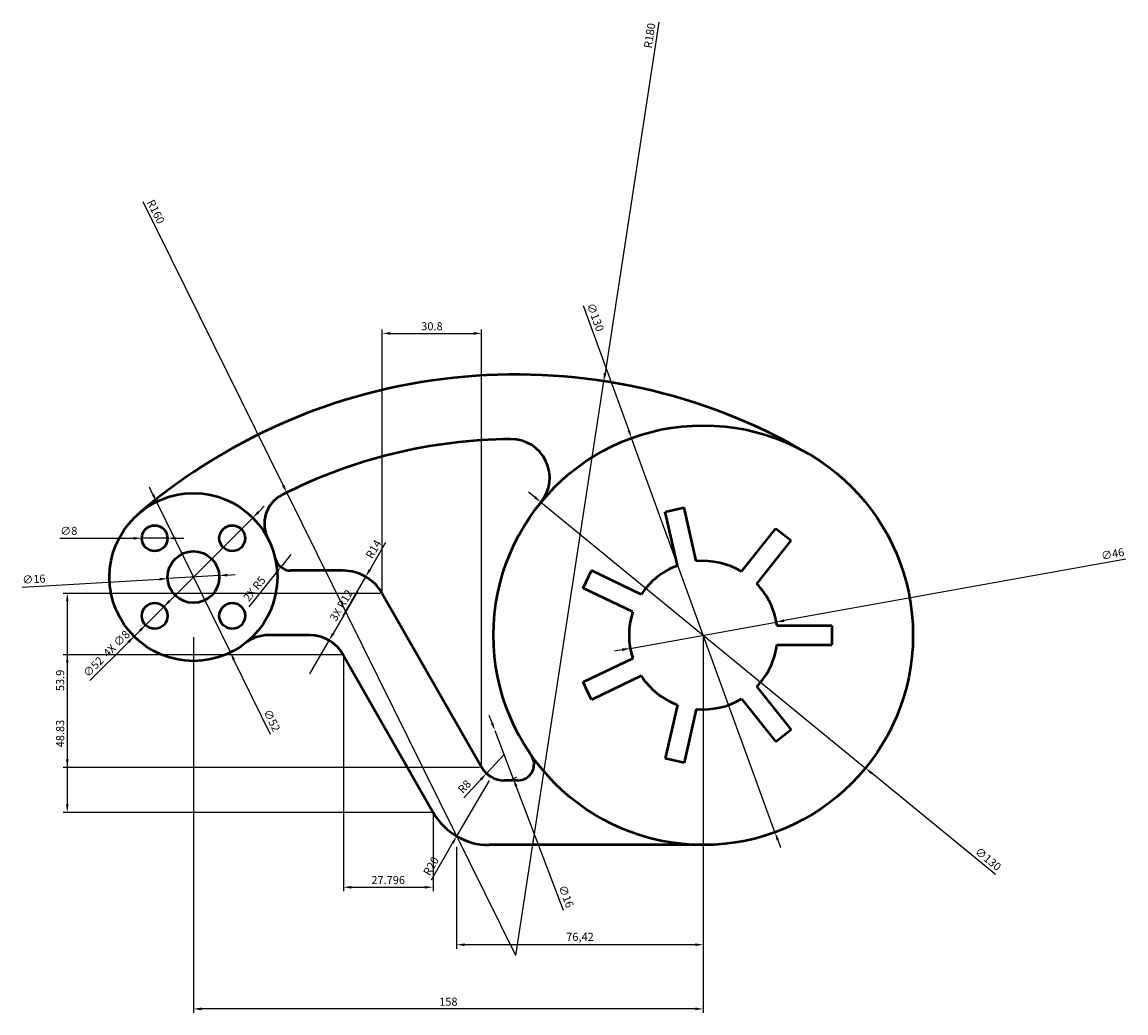
# Model space of a CAD drawing. Units: millimetres. Extents: x 750 to 1092, y 797 to 1104.
import ezdxf

# ---------------------------------------------------------------- set-up
doc = ezdxf.new("R2010")
doc.units = ezdxf.units.MM
doc.layers.add('M-DIMS', color=1, linetype='Continuous', lineweight=25)
doc.layers.add('M-OUTL', color=7, linetype='Continuous', lineweight=50)
doc.styles.get("Standard").update_dxf_attribs({"font": 'arial.ttf'})
doc.dimstyles.new('ISO-25', dxfattribs={"dimtxt": 2.5, "dimasz": 2.5, "dimexe": 1.25, "dimexo": 0.625, "dimtad": 1, "dimtxsty": 'Standard', "dimcen": 2.5, "dimadec": 0, "dimazin": 0, "dimtfac": 1, "dimtmove": 0, "dimatfit": 3, "dimfxl": 1, "dimarcsym": 0})

# ---------------------------------------------------------------- blocks, each defined once
blk = doc.blocks.new('*U1')
for p, q in [((-8.54, 3), (8.54, 3)), ((8.54, 3), (8.54, -3)), ((-8.54, -3), (8.54, -3))]:
    blk.add_line(p, q)
blk = doc.blocks.new('*U2')
at = {"layer": 'M-OUTL', "color": 0, "linetype": 'ByBlock', "lineweight": -2, "transparency": 16777216}
for p, rotation in [((4314.2, 1845.1), 102.8571428571428), ((4340.72, 1839.05), 51.4285714285714), ((4292.93, 1828.14), 154.2857142857142), ((4292.93, 1800.94), 205.7142857142856), ((4340.72, 1790.04), 308.5714285714284), ((4314.2, 1783.98), 257.1428571428571)]:
    blk.add_blockref('*U1', p, dxfattribs=dict(at, rotation=rotation))
blk.add_blockref('*U1', (4352.52, 1814.54), dxfattribs=at)
blk = doc.blocks.new('*D3')
at = {"layer": 'Defpoints', "color": 0, "transparency": 16777216}
for p in [(910.49, 955.31), (1011.06, 872.94)]:
    blk.add_point(p, dxfattribs=at)
at = {"layer": 'M-DIMS', "color": 0, "lineweight": -2, "transparency": 16777216}
for p, q in [((908.56, 956.9), (906.62, 958.48)), ((910.49, 955.31), (1011.06, 872.94)), ((1051.3, 839.99), (1013, 871.36))]:
    blk.add_line(p, q, dxfattribs=at)
at = {"layer": 'M-DIMS', "color": 0, "transparency": 16777216}
for points in [[(908.82, 957.22), (908.29, 956.57), (910.49, 955.31)], [(1013.26, 871.68), (1012.73, 871.04), (1011.06, 872.94)]]:
    blk.add_solid(points, dxfattribs=at)
at = {"layer": 'M-DIMS', "color": 0, "transparency": 16777216, "insert": (1048.88, 844.52), "char_height": 2.5, "attachment_point": 5, "rotation": 320.682}
blk.add_mtext('∅130', dxfattribs=at)
blk = doc.blocks.new('*D4')
at = {"layer": 'Defpoints', "color": 0, "transparency": 16777216}
for p in [(983.41, 918.2), (938.14, 910.05)]:
    blk.add_point(p, dxfattribs=at)
at = {"layer": 'M-DIMS', "color": 0, "lineweight": -2, "transparency": 16777216}
for p, q in [((1091.77, 937.72), (985.87, 918.65)), ((938.14, 910.05), (983.41, 918.2)), ((935.68, 909.61), (933.22, 909.16))]:
    blk.add_line(p, q, dxfattribs=at)
at = {"layer": 'M-DIMS', "color": 0, "transparency": 16777216}
for points in [[(985.8, 919.06), (985.95, 918.24), (983.41, 918.2)], [(935.61, 910.02), (935.76, 909.2), (938.14, 910.05)]]:
    blk.add_solid(points, dxfattribs=at)
at = {"layer": 'M-DIMS', "color": 0, "transparency": 16777216, "insert": (1087.71, 938.99), "char_height": 2.5, "attachment_point": 5, "rotation": 10.2107}
blk.add_mtext('∅46', dxfattribs=at)
blk = doc.blocks.new('*D5')
at = {"layer": 'Defpoints', "color": 0, "transparency": 16777216}
for p in [(791.34, 955.48), (814.21, 908.78)]:
    blk.add_point(p, dxfattribs=at)
at = {"layer": 'M-DIMS', "color": 0, "lineweight": -2, "transparency": 16777216}
for p, q in [((790.24, 957.72), (789.14, 959.97)), ((791.34, 955.48), (814.21, 908.78)), ((826.68, 883.32), (815.31, 906.53))]:
    blk.add_line(p, q, dxfattribs=at)
at = {"layer": 'M-DIMS', "color": 0, "transparency": 16777216}
for points in [[(790.61, 957.9), (789.87, 957.54), (791.34, 955.48)], [(815.69, 906.72), (814.94, 906.35), (814.21, 908.78)]]:
    blk.add_solid(points, dxfattribs=at)
at = {"layer": 'M-DIMS', "color": 0, "transparency": 16777216, "insert": (826.8, 887.57), "char_height": 2.5, "attachment_point": 5, "rotation": 296.098}
blk.add_mtext('∅52', dxfattribs=at)
blk = doc.blocks.new('*D6')
at = {"layer": 'Defpoints', "color": 0, "transparency": 16777216}
for p in [(794.79, 931.65), (810.76, 932.6)]:
    blk.add_point(p, dxfattribs=at)
at = {"layer": 'M-DIMS', "color": 0, "lineweight": -2, "transparency": 16777216}
for p, q in [((749.7, 928.97), (792.3, 931.5)), ((810.76, 932.6), (794.79, 931.65)), ((813.26, 932.75), (815.75, 932.9))]:
    blk.add_line(p, q, dxfattribs=at)
at = {"layer": 'M-DIMS', "color": 0, "transparency": 16777216}
for points in [[(792.27, 931.92), (792.32, 931.09), (794.79, 931.65)], [(813.23, 933.17), (813.28, 932.33), (810.76, 932.6)]]:
    blk.add_solid(points, dxfattribs=at)
at = {"layer": 'M-DIMS', "color": 0, "transparency": 16777216, "insert": (753.35, 931.16), "char_height": 2.5, "attachment_point": 5, "rotation": 3.4043}
blk.add_mtext('∅16', dxfattribs=at)
blk = doc.blocks.new('*D7')
at = {"layer": 'Defpoints', "color": 0, "transparency": 16777216}
for p in [(786.76, 944.15), (794.76, 944.15)]:
    blk.add_point(p, dxfattribs=at)
at = {"layer": 'M-DIMS', "color": 0, "lineweight": -2, "transparency": 16777216}
for p, q in [((761.33, 944.15), (784.26, 944.15)), ((794.76, 944.15), (786.76, 944.15)), ((797.26, 944.15), (799.76, 944.15))]:
    blk.add_line(p, q, dxfattribs=at)
at = {"layer": 'M-DIMS', "color": 0, "transparency": 16777216}
for points in [[(784.26, 944.56), (784.26, 943.73), (786.76, 944.15)], [(797.26, 944.56), (797.26, 943.73), (794.76, 944.15)]]:
    blk.add_solid(points, dxfattribs=at)
at = {"layer": 'M-DIMS', "color": 0, "transparency": 16777216, "insert": (764.14, 946.12), "char_height": 2.5, "attachment_point": 5}
blk.add_mtext('∅8', dxfattribs=at)
blk = doc.blocks.new('*D8')
at = {"layer": 'Defpoints', "color": 0, "transparency": 16777216}
for p in [(896.2, 884.6), (901.91, 869.65)]:
    blk.add_point(p, dxfattribs=at)
at = {"layer": 'M-DIMS', "color": 0, "lineweight": -2, "transparency": 16777216}
for p, q in [((895.31, 886.94), (894.42, 889.27)), ((896.2, 884.6), (901.91, 869.65)), ((917.51, 828.84), (902.81, 867.32))]:
    blk.add_line(p, q, dxfattribs=at)
blk.add_arc((899.06, 877.13), 8, 274.4762, 299.8708, dxfattribs=at)
at = {"layer": 'M-DIMS', "color": 0, "transparency": 16777216}
for points in [[(895.7, 887.08), (894.92, 886.79), (896.2, 884.6)], [(903.2, 867.47), (902.42, 867.17), (901.91, 869.65)]]:
    blk.add_solid(points, dxfattribs=at)
at = {"layer": 'M-DIMS', "color": 0, "transparency": 16777216, "insert": (918.01, 833.07), "char_height": 2.5, "attachment_point": 5, "rotation": 290.9183}
blk.add_mtext('∅16', dxfattribs=at)
blk = doc.blocks.new('*D9')
at = {"layer": 'Defpoints', "color": 0, "transparency": 16777216}
for p in [(802.78, 914.13), (960.78, 914.13), (802.78, 798.34)]:
    blk.add_point(p, dxfattribs=at)
at = {"layer": 'M-DIMS', "color": 0, "lineweight": -2, "transparency": 16777216}
for p, q in [((802.78, 913.5), (802.78, 797.09)), ((960.78, 913.5), (960.78, 797.09)), ((958.28, 798.34), (805.28, 798.34))]:
    blk.add_line(p, q, dxfattribs=at)
at = {"layer": 'M-DIMS', "color": 0, "transparency": 16777216}
for points in [[(805.28, 798.76), (805.28, 797.92), (802.78, 798.34)], [(958.28, 798.76), (958.28, 797.92), (960.78, 798.34)]]:
    blk.add_solid(points, dxfattribs=at)
at = {"layer": 'M-DIMS', "color": 0, "transparency": 16777216, "insert": (881.78, 800.24), "char_height": 2.5, "attachment_point": 5}
blk.add_mtext('158', dxfattribs=at)
blk = doc.blocks.new('*D10')
at = {"layer": 'Defpoints', "color": 0, "transparency": 16777216}
for p in [(884.35, 849.13), (960.78, 849.13), (884.35, 818.22)]:
    blk.add_point(p, dxfattribs=at)
at = {"layer": 'M-DIMS', "color": 0, "lineweight": -2, "transparency": 16777216}
for p, q in [((884.35, 848.5), (884.35, 816.97)), ((960.78, 848.5), (960.78, 816.97)), ((958.28, 818.22), (886.85, 818.22))]:
    blk.add_line(p, q, dxfattribs=at)
at = {"layer": 'M-DIMS', "color": 0, "transparency": 16777216}
for points in [[(886.85, 818.64), (886.85, 817.8), (884.35, 818.22)], [(958.28, 818.64), (958.28, 817.8), (960.78, 818.22)]]:
    blk.add_solid(points, dxfattribs=at)
at = {"layer": 'M-DIMS', "color": 0, "transparency": 16777216, "insert": (922.57, 820.35), "char_height": 2.5, "attachment_point": 5}
blk.add_mtext('76,42', dxfattribs=at)
blk = doc.blocks.new('*D11')
at = {"layer": 'Defpoints', "color": 0, "transparency": 16777216}
for p in [(849.23, 908.06), (877.02, 859.23), (877.02, 836.03)]:
    blk.add_point(p, dxfattribs=at)
at = {"layer": 'M-DIMS', "color": 0, "lineweight": -2, "transparency": 16777216}
for p, q in [((849.23, 907.44), (849.23, 834.78)), ((877.02, 858.61), (877.02, 834.78)), ((851.73, 836.03), (874.52, 836.03))]:
    blk.add_line(p, q, dxfattribs=at)
at = {"layer": 'M-DIMS', "color": 0, "transparency": 16777216}
for points in [[(851.73, 836.44), (851.73, 835.61), (849.23, 836.03)], [(874.52, 836.44), (874.52, 835.61), (877.02, 836.03)]]:
    blk.add_solid(points, dxfattribs=at)
at = {"layer": 'M-DIMS', "color": 0, "transparency": 16777216, "insert": (863.13, 837.93), "char_height": 2.5, "attachment_point": 5}
blk.add_mtext('27.796', dxfattribs=at)
blk = doc.blocks.new('*D12')
at = {"layer": 'Defpoints', "color": 0, "transparency": 16777216}
for p in [(849.23, 908.06), (763.68, 859.23), (877.02, 859.23)]:
    blk.add_point(p, dxfattribs=at)
at = {"layer": 'M-DIMS', "color": 0, "lineweight": -2, "transparency": 16777216}
for p, q in [((848.6, 908.06), (762.43, 908.06)), ((763.68, 905.56), (763.68, 861.73)), ((876.4, 859.23), (762.43, 859.23))]:
    blk.add_line(p, q, dxfattribs=at)
at = {"layer": 'M-DIMS', "color": 0, "transparency": 16777216}
for points in [[(763.26, 905.56), (764.09, 905.56), (763.68, 908.06)], [(763.26, 861.73), (764.09, 861.73), (763.68, 859.23)]]:
    blk.add_solid(points, dxfattribs=at)
at = {"layer": 'M-DIMS', "color": 0, "transparency": 16777216, "insert": (761.78, 883.65), "char_height": 2.5, "attachment_point": 5, "rotation": 90}
blk.add_mtext('48.83', dxfattribs=at)
blk = doc.blocks.new('*D13')
at = {"layer": 'Defpoints', "color": 0, "transparency": 16777216}
for p in [(892.1, 1007.63), (861.3, 927.07), (892.1, 873.17)]:
    blk.add_point(p, dxfattribs=at)
at = {"layer": 'M-DIMS', "color": 0, "lineweight": -2, "transparency": 16777216}
for p, q in [((861.3, 927.7), (861.3, 1008.88)), ((863.8, 1007.63), (889.6, 1007.63)), ((892.1, 873.79), (892.1, 1008.88))]:
    blk.add_line(p, q, dxfattribs=at)
at = {"layer": 'M-DIMS', "color": 0, "transparency": 16777216}
for points in [[(863.8, 1008.05), (863.8, 1007.21), (861.3, 1007.63)], [(889.6, 1008.05), (889.6, 1007.21), (892.1, 1007.63)]]:
    blk.add_solid(points, dxfattribs=at)
at = {"layer": 'M-DIMS', "color": 0, "transparency": 16777216, "insert": (876.7, 1009.53), "char_height": 2.5, "attachment_point": 5}
blk.add_mtext('30.8', dxfattribs=at)
blk = doc.blocks.new('*D14')
at = {"layer": 'Defpoints', "color": 0, "transparency": 16777216}
for p in [(861.3, 927.07), (763.68, 873.17), (892.1, 873.17)]:
    blk.add_point(p, dxfattribs=at)
at = {"layer": 'M-DIMS', "color": 0, "lineweight": -2, "transparency": 16777216}
for p, q in [((860.68, 927.07), (762.43, 927.07)), ((763.68, 924.57), (763.68, 875.67)), ((891.48, 873.17), (762.43, 873.17))]:
    blk.add_line(p, q, dxfattribs=at)
at = {"layer": 'M-DIMS', "color": 0, "transparency": 16777216}
for points in [[(763.26, 924.57), (764.09, 924.57), (763.68, 927.07)], [(763.26, 875.67), (764.09, 875.67), (763.68, 873.17)]]:
    blk.add_solid(points, dxfattribs=at)
at = {"layer": 'M-DIMS', "color": 0, "transparency": 16777216, "insert": (761.78, 900.12), "char_height": 2.5, "attachment_point": 5, "rotation": 90}
blk.add_mtext('53.9', dxfattribs=at)
blk = doc.blocks.new('*D15')
at = {"layer": 'Defpoints', "color": 0, "transparency": 16777216}
for p in [(929.97, 992.81), (902.65, 814.9)]:
    blk.add_point(p, dxfattribs=at)
at = {"layer": 'M-DIMS', "color": 0, "lineweight": -2, "transparency": 16777216}
for p, q in [((947.06, 1104.09), (930.35, 995.29)), ((902.65, 814.9), (929.97, 992.81))]:
    blk.add_line(p, q, dxfattribs=at)
at = {"layer": 'M-DIMS', "color": 0, "transparency": 16777216}
blk.add_solid([(929.94, 995.35), (930.76, 995.22), (929.97, 992.81)], dxfattribs=at)
at = {"layer": 'M-DIMS', "color": 0, "transparency": 16777216, "insert": (944.49, 1099.85), "char_height": 2.5, "attachment_point": 5, "rotation": 81.2686}
blk.add_mtext('R180', dxfattribs=at)
blk = doc.blocks.new('*D16')
at = {"layer": 'Defpoints', "color": 0, "transparency": 16777216}
for p in [(831.69, 958.31), (902.65, 814.9)]:
    blk.add_point(p, dxfattribs=at)
at = {"layer": 'M-DIMS', "color": 0, "lineweight": -2, "transparency": 16777216}
for p, q in [((787.09, 1048.46), (830.59, 960.55)), ((902.65, 814.9), (831.69, 958.31))]:
    blk.add_line(p, q, dxfattribs=at)
at = {"layer": 'M-DIMS', "color": 0, "transparency": 16777216}
blk.add_solid([(830.96, 960.73), (830.21, 960.36), (831.69, 958.31)], dxfattribs=at)
at = {"layer": 'M-DIMS', "color": 0, "transparency": 16777216, "insert": (790.83, 1045.2), "char_height": 2.5, "attachment_point": 5, "rotation": 296.3247}
blk.add_mtext('R160', dxfattribs=at)
blk = doc.blocks.new('*D17')
at = {"layer": 'Defpoints', "color": 0, "transparency": 16777216}
for p in [(894.41, 869.13), (884.35, 851.84)]:
    blk.add_point(p, dxfattribs=at)
at = {"layer": 'M-DIMS', "color": 0, "lineweight": -2, "transparency": 16777216}
for p, q in [((894.41, 869.13), (884.35, 851.84)), ((876.51, 838.34), (883.1, 849.68))]:
    blk.add_line(p, q, dxfattribs=at)
at = {"layer": 'M-DIMS', "color": 0, "transparency": 16777216}
blk.add_solid([(882.74, 849.89), (883.46, 849.47), (884.35, 851.84)], dxfattribs=at)
at = {"layer": 'M-DIMS', "color": 0, "transparency": 16777216, "insert": (876.68, 842.42), "char_height": 2.5, "attachment_point": 5, "rotation": 59.8252}
blk.add_mtext('R20', dxfattribs=at)
blk = doc.blocks.new('*D18')
at = {"layer": 'Defpoints', "color": 0, "transparency": 16777216}
for p in [(856.17, 932.24), (849.15, 920.13)]:
    blk.add_point(p, dxfattribs=at)
at = {"layer": 'M-DIMS', "color": 0, "lineweight": -2, "transparency": 16777216}
for p, q in [((862.3, 942.8), (857.43, 934.4)), ((849.15, 920.13), (856.17, 932.24))]:
    blk.add_line(p, q, dxfattribs=at)
at = {"layer": 'M-DIMS', "color": 0, "transparency": 16777216}
blk.add_solid([(857.07, 934.61), (857.79, 934.19), (856.17, 932.24)], dxfattribs=at)
at = {"layer": 'M-DIMS', "color": 0, "transparency": 16777216, "insert": (858.87, 940.62), "char_height": 2.5, "attachment_point": 5, "rotation": 59.8719}
blk.add_mtext('R14', dxfattribs=at)
blk = doc.blocks.new('*D19')
at = {"layer": 'Defpoints', "color": 0, "transparency": 16777216}
for p in [(844.83, 912.5), (838.8, 902.13)]:
    blk.add_point(p, dxfattribs=at)
at = {"layer": 'M-DIMS', "color": 0, "lineweight": -2, "transparency": 16777216}
for p, q in [((853.66, 927.69), (846.09, 914.66)), ((838.8, 902.13), (844.83, 912.5))]:
    blk.add_line(p, q, dxfattribs=at)
at = {"layer": 'M-DIMS', "color": 0, "transparency": 16777216}
blk.add_solid([(845.73, 914.87), (846.45, 914.45), (844.83, 912.5)], dxfattribs=at)
at = {"layer": 'M-DIMS', "color": 0, "transparency": 16777216, "insert": (848.86, 923.21), "char_height": 2.5, "attachment_point": 5, "rotation": 59.8241}
blk.add_mtext('3X R12', dxfattribs=at)
blk = doc.blocks.new('*D20')
at = {"layer": 'Defpoints', "color": 0, "transparency": 16777216}
for p in [(832.98, 939.13), (829.87, 935.21)]:
    blk.add_point(p, dxfattribs=at)
at = {"layer": 'M-DIMS', "color": 0, "lineweight": -2, "transparency": 16777216}
for p, q in [((832.98, 939.13), (829.87, 935.21)), ((820.09, 922.91), (828.31, 933.26))]:
    blk.add_line(p, q, dxfattribs=at)
at = {"layer": 'M-DIMS', "color": 0, "transparency": 16777216}
blk.add_solid([(827.98, 933.51), (828.64, 933), (829.87, 935.21)], dxfattribs=at)
at = {"layer": 'M-DIMS', "color": 0, "transparency": 16777216, "insert": (821.93, 928.29), "char_height": 2.5, "attachment_point": 5, "rotation": 51.5253}
blk.add_mtext('2X R5', dxfattribs=at)
blk = doc.blocks.new('*D21')
at = {"layer": 'Defpoints', "color": 0, "transparency": 16777216}
for p in [(899.06, 877.13), (893.6, 871.28)]:
    blk.add_point(p, dxfattribs=at)
at = {"layer": 'M-DIMS', "color": 0, "lineweight": -2, "transparency": 16777216}
for p, q in [((899.06, 877.13), (893.6, 871.28)), ((886.57, 863.77), (891.89, 869.45))]:
    blk.add_line(p, q, dxfattribs=at)
at = {"layer": 'M-DIMS', "color": 0, "transparency": 16777216}
blk.add_solid([(891.58, 869.74), (892.19, 869.17), (893.6, 871.28)], dxfattribs=at)
at = {"layer": 'M-DIMS', "color": 0, "transparency": 16777216, "insert": (886.99, 866.99), "char_height": 2.5, "attachment_point": 5, "rotation": 46.9458}
blk.add_mtext('R8', dxfattribs=at)
blk = doc.blocks.new('*D22')
at = {"layer": 'Defpoints', "color": 0, "transparency": 16777216}
for p in [(821.16, 950.51), (784.39, 913.74)]:
    blk.add_point(p, dxfattribs=at)
at = {"layer": 'M-DIMS', "color": 0, "lineweight": -2, "transparency": 16777216}
for p, q in [((822.93, 952.28), (824.7, 954.05)), ((821.16, 950.51), (784.39, 913.74)), ((770.7, 900.05), (782.62, 911.97))]:
    blk.add_line(p, q, dxfattribs=at)
at = {"layer": 'M-DIMS', "color": 0, "transparency": 16777216}
for points in [[(822.64, 952.57), (823.22, 951.99), (821.16, 950.51)], [(782.33, 912.27), (782.92, 911.68), (784.39, 913.74)]]:
    blk.add_solid(points, dxfattribs=at)
at = {"layer": 'M-DIMS', "color": 0, "transparency": 16777216, "insert": (771.97, 904.11), "char_height": 2.5, "attachment_point": 5, "rotation": 44.9998}
blk.add_mtext('∅52', dxfattribs=at)
blk = doc.blocks.new('*D23')
at = {"layer": 'Defpoints', "color": 0, "transparency": 16777216}
for p in [(793.59, 922.93), (787.93, 917.28)]:
    blk.add_point(p, dxfattribs=at)
at = {"layer": 'M-DIMS', "color": 0, "lineweight": -2, "transparency": 16777216}
for p, q in [((795.35, 924.7), (797.12, 926.47)), ((793.59, 922.93), (787.93, 917.28)), ((776.65, 906), (786.16, 915.51))]:
    blk.add_line(p, q, dxfattribs=at)
at = {"layer": 'M-DIMS', "color": 0, "transparency": 16777216}
for points in [[(795.06, 925), (795.65, 924.41), (793.59, 922.93)], [(785.87, 915.8), (786.45, 915.22), (787.93, 917.28)]]:
    blk.add_solid(points, dxfattribs=at)
at = {"layer": 'M-DIMS', "color": 0, "transparency": 16777216, "insert": (779.13, 911.26), "char_height": 2.5, "attachment_point": 5, "rotation": 44.9986}
blk.add_mtext('4X ∅8', dxfattribs=at)
blk = doc.blocks.new('*D24')
at = {"layer": 'Defpoints', "color": 0, "transparency": 16777216}
for p in [(938.55, 975.21), (983.01, 853.05)]:
    blk.add_point(p, dxfattribs=at)
at = {"layer": 'M-DIMS', "color": 0, "lineweight": -2, "transparency": 16777216}
for p, q in [((923.59, 1016.31), (937.69, 977.56)), ((983.01, 853.05), (938.55, 975.21)), ((983.86, 850.7), (984.72, 848.35))]:
    blk.add_line(p, q, dxfattribs=at)
at = {"layer": 'M-DIMS', "color": 0, "transparency": 16777216}
for points in [[(938.08, 977.7), (937.3, 977.41), (938.55, 975.21)], [(984.25, 850.84), (983.47, 850.55), (983.01, 853.05)]]:
    blk.add_solid(points, dxfattribs=at)
at = {"layer": 'M-DIMS', "color": 0, "transparency": 16777216, "insert": (927.06, 1012.53), "char_height": 2.5, "attachment_point": 5, "rotation": 289.9989}
blk.add_mtext('∅130', dxfattribs=at)

msp = doc.modelspace()

# ---------------------------------------------------------------- linework, layer by layer
at = {"layer": 'M-OUTL'}
for p, q in [((849.1468, 934.1272), (832.9767, 934.1272)), ((861.3022, 927.0732), (892.1049, 873.1696)), ((838.8001, 914.1272), (826.1011, 914.1272)), ((849.2289, 908.0636), (877.0247, 859.2332)), ((903.3317, 869.1272), (899.0574, 869.1272)), ((960.7773, 849.1272), (894.406, 849.1272))]:
    msp.add_line(p, q, dxfattribs=at)
for centre, radius in [((960.7773, 914.1272), 65), ((802.7773, 932.1272), 26), ((790.7565, 944.148), 4), ((814.7981, 944.148), 4), ((802.7773, 932.1272), 8), ((790.7565, 920.1064), 4), ((814.7981, 920.1064), 4)]:
    msp.add_circle(centre, radius, dxfattribs=at)
for centre, radius, start, end in [((902.6471, 814.9008), 180, 59.636766, 130.428984), ((902.6471, 814.9008), 160, 90.564711, 116.910454), ((901.1884, 962.8936), 12, 320.703759, 90.564711), ((834.7575, 948.658), 10, 116.910454, 207.334871), ((832.9767, 939.1272), 5, 193.050305, 270), ((849.1468, 920.1272), 14, 29.745402, 90), ((960.7773, 914.1272), 23, 110.35186, 146.790997), ((960.7773, 914.1272), 23, 58.923289, 95.362425), ((960.7773, 914.1272), 23, 7.494717, 43.933854), ((960.7773, 914.1272), 23, 161.780432, 198.219568), ((826.1011, 902.1272), 12, 90, 127.863646), ((838.8001, 902.1272), 12, 29.649864, 90), ((960.7773, 914.1272), 23, 316.066146, 352.505283), ((960.7773, 914.1272), 23, 213.209003, 249.64814), ((960.7773, 914.1272), 23, 264.637575, 301.076711), ((903.3317, 874.1272), 5, 270, 34.849905), ((899.0574, 877.1272), 8, 209.649864, 270), ((894.406, 869.1272), 20, 209.649864, 270)]:
    msp.add_arc(centre, radius, start, end, dxfattribs=at)

# ---------------------------------------------------------------- block references
msp.add_blockref('*U2', (-3360.3972, -900.4157), dxfattribs=at)

# ---------------------------------------------------------------- dimensions: what is measured, and where the dimension line sits
at = {"layer": 'M-DIMS'}
for center, mpoint, picture, middle in [((902.6471, 814.9008), (929.9715, 992.8147), '*D15', (946.3662, 1099.5631)), ((902.6471, 814.9008), (831.6939, 958.3081), '*D16', (789.122, 1044.3524)), ((894.406, 869.1272), (884.3532, 851.8373), '*D17', (878.3215, 841.4633))]:
    dim = msp.add_radius_dim(center=center, mpoint=mpoint, dimstyle='ISO-25', override={"dimdec": 0, "dimlfac": 1, "dimrnd": 0, "dimzin": 0, "dimdsep": 46, "dimlunit": 2}, dxfattribs=at)
    dim.commit()
    dim.dimension.update_dxf_attribs({"geometry": picture, "text_midpoint": middle, "dimtype": 164})
for p1, p2, override, picture, middle in [((983.0074, 853.0467), (938.5472, 975.2076), {"dimdec": 0, "dimlfac": 1, "dimrnd": 0, "dimzin": 0, "dimdsep": 46, "dimlunit": 2}, '*D24', (925.2092, 1011.8559)), ((791.3397, 955.4763), (814.2149, 908.7781), {"dimclrd": 0, "dimclre": 0, "dimclrt": 0}, '*D5', (825.0288, 886.7024)), ((910.4907, 955.3128), (1011.064, 872.9416), {"dimclrd": 0, "dimclre": 0, "dimclrt": 0}, '*D3', (1047.6321, 842.9917)), ((821.1622, 950.5119), (784.3925, 913.7425), {"dimdec": 0, "dimlfac": 1, "dimrnd": 0, "dimzin": 0, "dimdsep": 46, "dimlunit": 2}, '*D22', (773.3616, 902.7117)), ((794.7565, 944.148), (786.7565, 944.148), {"dimclrd": 0, "dimclre": 0, "dimclrt": 0}, '*D7', (764.1405, 944.148)), ((938.1416, 910.05), (983.4131, 918.2044), {"dimclrd": 0, "dimclre": 0, "dimclrt": 0}, '*D4', (1088.0551, 937.0527)), ((810.7632, 932.6022), (794.7914, 931.6521), {"dimclrd": 0, "dimclre": 0, "dimclrt": 0}, '*D6', (753.472, 929.1942)), ((896.2011, 884.5999), (901.9137, 869.6545), {"dimclrd": 0, "dimclre": 0, "dimclrt": 0}, '*D8', (916.1666, 832.3656))]:
    dim = msp.add_diameter_dim_2p(p1=p1, p2=p2, dimstyle='ISO-25', override=override, dxfattribs=at)
    dim.commit()
    dim.dimension.update_dxf_attribs({"geometry": picture, "text_midpoint": middle, "dimtype": 163})
for base, p1, p2, override, picture, middle in [((892.1049, 1007.6312), (861.3022, 927.0732), (892.1049, 873.1696), {"dimdec": 1, "dimlfac": 1, "dimrnd": 0, "dimzin": 0, "dimdsep": 46, "dimlunit": 2}, '*D13', (876.7035, 1009.5335)), ((877.0247, 836.0272), (849.2289, 908.0636), (877.0247, 859.2332), {"dimdec": 3, "dimlfac": 1, "dimrnd": 0, "dimzin": 0, "dimdsep": 46, "dimlunit": 2}, '*D11', (863.1268, 837.9286))]:
    dim = msp.add_linear_dim(base=base, p1=p1, p2=p2, dimstyle='ISO-25', override=override, dxfattribs=at)
    dim.commit()
    dim.dimension.update_dxf_attribs({"geometry": picture, "text_midpoint": middle})
for center, mpoint, picture, middle in [((849.1468, 920.1272), (856.1739, 932.2359), '*D18', (858.8678, 940.6236)), ((899.0574, 877.1272), (893.5959, 871.2815), '*D21', (886.9885, 866.9946))]:
    dim = msp.add_radius_dim(center=center, mpoint=mpoint, dimstyle='ISO-25', override={"dimdec": 0, "dimlfac": 1, "dimrnd": 0, "dimzin": 0, "dimdsep": 46, "dimlunit": 2}, dxfattribs=at)
    dim.commit()
    dim.dimension.update_dxf_attribs({"geometry": picture, "text_midpoint": middle})
for center, mpoint, text, picture, middle in [((832.9767, 939.1272), (829.8658, 935.2128), '2X <>', '*D20', (821.9333, 928.2873)), ((838.8001, 902.1272), (844.832, 912.501), '3X <>', '*D19', (848.8595, 923.2122))]:
    dim = msp.add_radius_dim(center=center, mpoint=mpoint, text=text, dimstyle='ISO-25', override={"dimdec": 0, "dimlfac": 1, "dimrnd": 0, "dimzin": 0, "dimdsep": 46, "dimlunit": 2}, dxfattribs=at)
    dim.commit()
    dim.dimension.update_dxf_attribs({"geometry": picture, "text_midpoint": middle})
for base, p1, p2, override, picture, middle in [((763.6773, 873.1696), (861.3022, 927.0732), (892.1049, 873.1696), {"dimdec": 1, "dimlfac": 1, "dimrnd": 0, "dimzin": 0, "dimdsep": 46, "dimlunit": 2}, '*D14', (761.775, 900.1214)), ((763.6773, 859.2332), (849.2289, 908.0636), (877.0247, 859.2332), {"dimdec": 2, "dimlfac": 1, "dimrnd": 0, "dimzin": 0, "dimdsep": 46, "dimlunit": 2}, '*D12', (761.775, 883.6484))]:
    dim = msp.add_linear_dim(base=base, p1=p1, p2=p2, angle=90, dimstyle='ISO-25', override=override, dxfattribs=at)
    dim.commit()
    dim.dimension.update_dxf_attribs({"geometry": picture, "text_midpoint": middle})
dim = msp.add_diameter_dim_2p(p1=(793.585, 922.9347), p2=(787.928, 917.278), text='4X <>', dimstyle='ISO-25', override={"dimdec": 0, "dimlfac": 1, "dimrnd": 0, "dimzin": 0, "dimdsep": 46, "dimlunit": 2}, dxfattribs=at)
dim.commit()
dim.dimension.update_dxf_attribs({"geometry": '*D23', "text_midpoint": (780.5197, 909.8701)})
for p1, p2, distance, picture, middle in [((960.7773, 914.1272), (802.7773, 914.1272), 115.7865, '*D9', (881.7773, 800.2421)), ((960.7773, 849.1272), (884.3531, 849.1272), 30.9084, '*D10', (922.5652, 820.3461))]:
    dim = msp.add_aligned_dim(p1=p1, p2=p2, distance=distance, dimstyle='ISO-25', override={"dimclrd": 0, "dimclre": 0, "dimclrt": 0}, dxfattribs=at)
    dim.commit()
    dim.dimension.update_dxf_attribs({"geometry": picture, "text_midpoint": middle})

doc.saveas('drawing.dxf')
